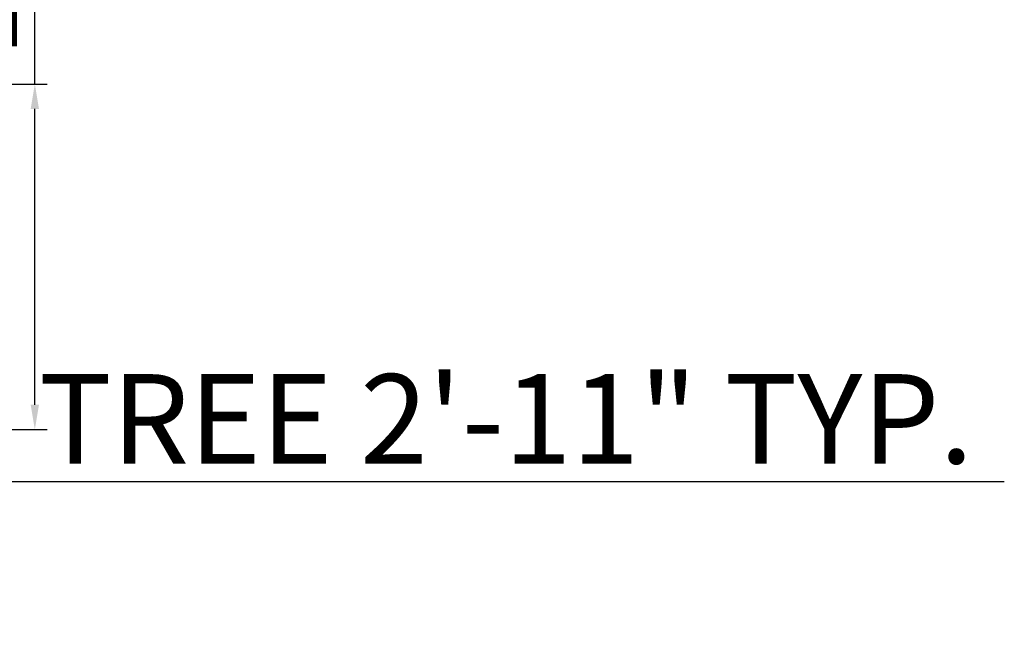
# Model space of a CAD drawing. Units: inches. Extents: x 2337 to 3570, y 1258 to 1938.
# Tile 29 of 30: x 3471 to 3570, y 1702 to 1764. Entities that reach past the tile are written whole.
import ezdxf

# ---------------------------------------------------------------- set-up
doc = ezdxf.new("R2010")
doc.units = ezdxf.units.IN
doc.layers.add('A-ANNO-DIMS', color=2, linetype='Continuous', lineweight=18)
doc.styles.get("Standard").update_dxf_attribs({"font": 'arial.ttf'})
doc.dimstyles.new('ISO-25', dxfattribs={"dimtxt": 9, "dimasz": 2.5, "dimexe": 1.25, "dimexo": 0.625, "dimtad": 1, "dimdec": 1, "dimlunit": 3, "dimtxsty": 'Standard', "dimcen": 2.5, "dimadec": 0, "dimazin": 0, "dimtfac": 1, "dimtdec": 1, "dimtmove": 0, "dimatfit": 3, "dimfxl": 1, "dimarcsym": 0})

# ---------------------------------------------------------------- blocks, each defined once
blk = doc.blocks.new('*D48')
at = {"layer": 'A-ANNO-DIMS', "color": 0, "lineweight": -2, "transparency": 16777216}
for p, q in [((3431.986, 1722.217), (3431.986, 1716.362)), ((3466.853, 1722.217), (3466.853, 1716.362)), ((3434.486, 1717.612), (3464.353, 1717.612)), ((3466.853, 1717.612), (3569.707, 1717.612))]:
    blk.add_line(p, q, dxfattribs=at)
at = {"layer": 'A-ANNO-DIMS', "color": 0, "transparency": 16777216}
for points in [[(3434.486, 1718.029), (3434.486, 1717.195), (3431.986, 1717.612)], [(3464.353, 1718.029), (3464.353, 1717.195), (3466.853, 1717.612)]]:
    blk.add_solid(points, dxfattribs=at)
at = {"layer": 'Defpoints', "color": 0, "transparency": 16777216}
for p in [(3431.986, 1722.842), (3466.853, 1722.842), (3466.853, 1717.612)]:
    blk.add_point(p, dxfattribs=at)
at = {"layer": 'A-ANNO-DIMS', "color": 0, "transparency": 16777216, "insert": (3519.53, 1722.759), "char_height": 9, "attachment_point": 5}
blk.add_mtext('TREE 2\'-11" TYP.', dxfattribs=at)
blk = doc.blocks.new('*D49')
at = {"layer": 'A-ANNO-DIMS', "color": 0, "lineweight": -2, "transparency": 16777216}
for p, q in [((3472.083, 1757.633), (3472.083, 1823.389)), ((3467.478, 1757.633), (3473.333, 1757.633)), ((3472.083, 1725.342), (3472.083, 1755.133)), ((3467.478, 1722.842), (3473.333, 1722.842))]:
    blk.add_line(p, q, dxfattribs=at)
at = {"layer": 'A-ANNO-DIMS', "color": 0, "transparency": 16777216}
for points in [[(3471.666, 1755.133), (3472.5, 1755.133), (3472.083, 1757.633)], [(3471.666, 1725.342), (3472.5, 1725.342), (3472.083, 1722.842)]]:
    blk.add_solid(points, dxfattribs=at)
at = {"layer": 'Defpoints', "color": 0, "transparency": 16777216}
for p in [(3466.853, 1757.633), (3472.083, 1757.633), (3466.853, 1722.842)]:
    blk.add_point(p, dxfattribs=at)
at = {"layer": 'A-ANNO-DIMS', "color": 0, "transparency": 16777216, "insert": (3466.936, 1791.761), "char_height": 9, "attachment_point": 5, "rotation": 90}
blk.add_mtext('2\'-11" TYP.', dxfattribs=at)

msp = doc.modelspace()

# ---------------------------------------------------------------- dimensions: what is measured, and where the dimension line sits
at = {"layer": 'A-ANNO-DIMS'}
dim = msp.add_linear_dim(base=(3472.083, 1757.633), p1=(3466.853, 1722.842), p2=(3466.853, 1757.633), angle=90, text='<> TYP.', dimstyle='ISO-25', override={"dimdec": 1, "dimlfac": 1, "dimrnd": 0, "dimzin": 1, "dimdsep": 46, "dimlunit": 4, "dimfrac": 2}, dxfattribs=at)
dim.commit()
dim.dimension.update_dxf_attribs({"geometry": '*D49', "text_midpoint": (3466.936, 1791.761)})
dim = msp.add_linear_dim(base=(3466.853, 1717.612), p1=(3431.986, 1722.842), p2=(3466.853, 1722.842), text='TREE <> TYP.', dimstyle='ISO-25', override={"dimdec": 1, "dimlfac": 1, "dimrnd": 0, "dimzin": 1, "dimdsep": 46, "dimlunit": 4, "dimfrac": 2}, dxfattribs=at)
dim.commit()
dim.dimension.update_dxf_attribs({"geometry": '*D48', "text_midpoint": (3519.53, 1722.759)})

doc.saveas('drawing.dxf')
